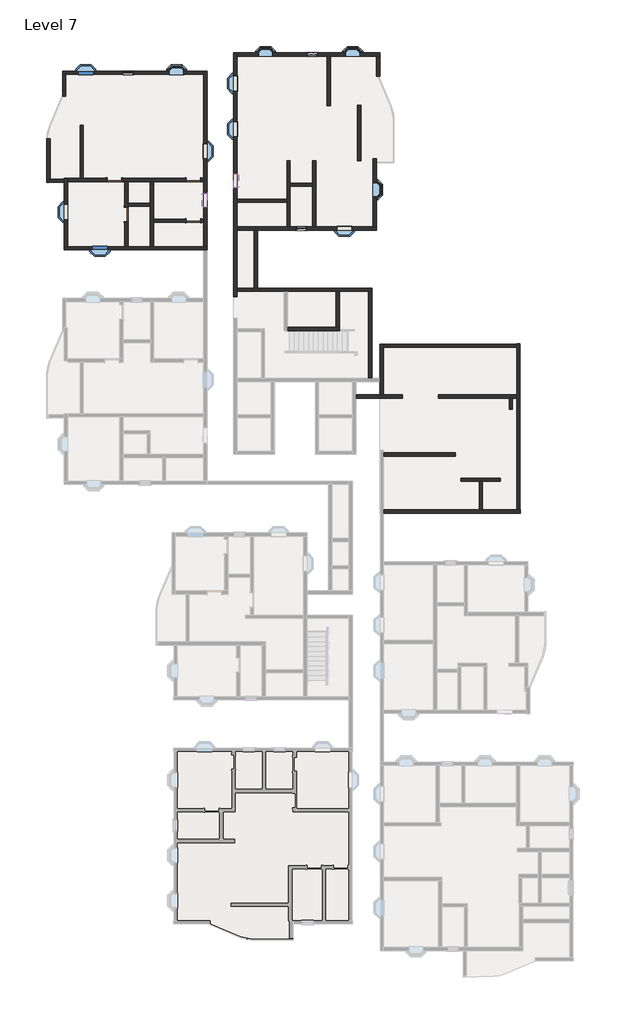
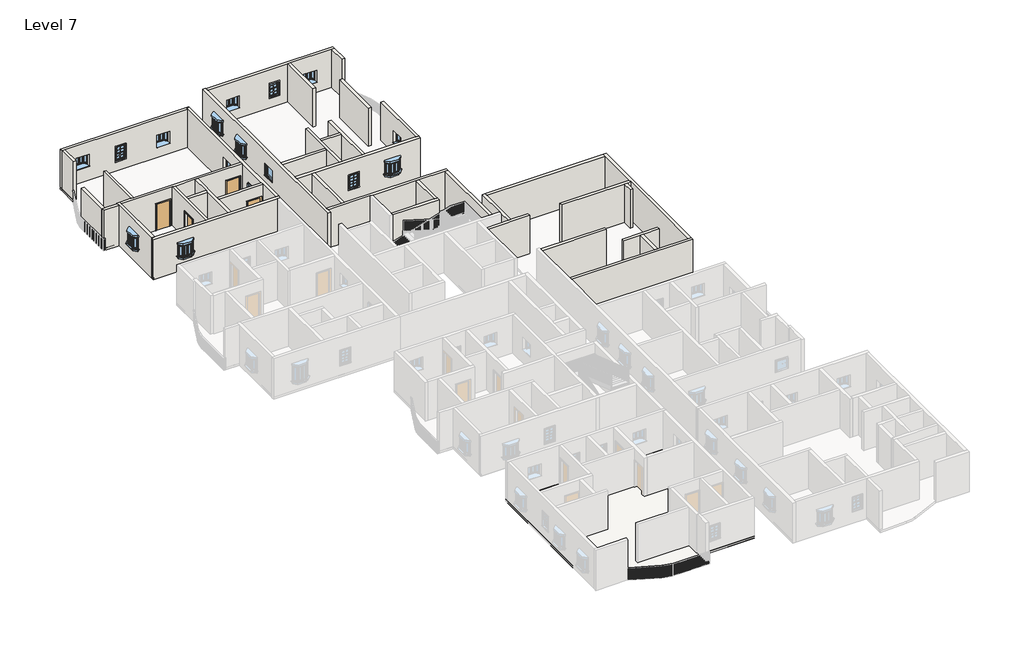
# One storey, part 4 of 14: 39 walls, 16 windows, 4 doors, 2 roofs.
# Revit data of these elements (continued)
# Elements 31, 45 (IfcWall, "9\" w") (continued)
#   wall height = 10' - 0"
#   Phase Created = New Construction
#   Base Constraint = Level 7
#   Top Constraint = Level 8
#   Materials on its faces: "Default Wall", "Brick, Soldier Course"
# Element 32 (IfcWall, "9\" w")
#   Top Offset = 0' - 0"
#   Base Offset = 0' - 0"
#   wall height = 10' - 0"
#   Phase Created = New Construction
#   Base Constraint = Level 7
#   Top Constraint = Level 8
#   Materials on its faces: "Default Wall", "Grass"
# Element 33 (IfcWall, "9\" w")
#   Top Offset = 0' - 0"
#   Base Offset = 0' - 0"
#   wall height = 10' - 0"
#   Phase Created = New Construction
#   Base Constraint = Level 7
#   Top Constraint = Level 8
#   Materials on its faces: "Default Wall", "Brick, Soldier Course", "Earth"
# Element 34 (IfcWall, "9\" w")
#   Top Offset = 0' - 0"
#   Base Offset = 0' - 0"
#   wall height = 10' - 0"
#   Phase Created = New Construction
#   Base Constraint = Level 7
#   Top Constraint = Level 8
#   Materials on its faces: "Default Wall", "Earth"
# Element 35 (IfcWall, "9\" w")
#   Top Offset = 0' - 0"
#   Base Offset = 0' - 0"
#   wall height = 10' - 0"
#   Phase Created = New Construction
#   Base Constraint = Level 7
#   Top Constraint = Level 8
#   Materials on its faces: "Default Wall", "Parking Stripe"
# Elements 36, 37, 38 (IfcWall, "9\" w")
#   Top Offset = 0' - 0"
#   Base Offset = 0' - 0"
#   wall height = 10' - 0"
#   Phase Created = New Construction
#   Base Constraint = Level 7
#   Top Constraint = Level 8
#   Materials on its faces: "Default Wall", "Window Frame"
# Element 43 (IfcWall, "9\" w")
#   Top Offset = 0' - 0"
#   Base Offset = 0' - 0"
#   wall height = 10' - 0"
#   Phase Created = New Construction
#   Base Constraint = Level 7
#   Top Constraint = Level 8
#   Materials on its faces: "Default Wall", "Parking Stripe", "Default Mass Interior Wall"
# Element 44 (IfcWall, "9\" w")
#   Top Offset = 0' - 0"
#   Base Offset = 0' - 0"
#   wall height = 10' - 0"
#   Phase Created = New Construction
#   Base Constraint = Level 7
#   Top Constraint = Level 8
#   Materials on its faces: "Default Wall", "Parking Stripe", "Brick, Soldier Course"
# Element 46 (IfcWindow, "910x910mm")
#   Mark = "362"
#   Phase Created = New Construction
#   Materials on its faces: "Window Frame", "Glass"
# Element 47 (IfcWindow, "910x910mm")
#   Mark = "363"
#   Phase Created = New Construction
#   Materials on its faces: "Window Frame", "Glass"
# Element 48 (IfcWindow, "910x910mm")
#   Mark = "364"
#   Phase Created = New Construction
#   Materials on its faces: "Window Frame", "Glass"
# Element 49 (IfcWindow, "910x910mm")
#   Mark = "394"
#   Phase Created = New Construction
#   Materials on its faces: "Window Frame", "Glass"
# Element 50 (IfcWindow, "910x910mm")
#   Mark = "395"
#   Phase Created = New Construction
#   Materials on its faces: "Window Frame", "Glass"
# Element 51 (IfcWindow, "910x910mm")
#   Mark = "475"
#   Phase Created = New Construction
#   Materials on its faces: "Window Frame", "Glass"
# Element 52 (IfcWindow, "910x910mm")
#   Mark = "476"
#   Phase Created = New Construction
#   Materials on its faces: "Window Frame", "Glass"
# Element 53 (IfcWindow, "910x910mm")
#   Mark = "484"
#   Phase Created = New Construction
#   Materials on its faces: "Window Frame", "Glass"
# Element 54 (IfcWindow, "910x910mm")
#   Mark = "485"
#   Phase Created = New Construction
#   Materials on its faces: "Window Frame", "Glass"
# Element 55 (IfcWindow, "910x910mm")
#   Mark = "396"
#   Phase Created = New Construction
#   Materials on its faces: "Window Frame", "Glass"
# Element 56 (IfcWindow, "910x910mm")
#   Mark = "397"
#   Phase Created = New Construction
#   Materials on its faces: "Window Frame", "Glass"
# Element 57 (IfcWindow, "Window-Double-Hung : 26\" x 42\"")
#   Mark = "477"
#   Window Inset = 0' - 0"
#   Interior Wall Closure = 0' - 1 1/2"
#   Frame Extension = 0' - 1 1/4"
#   Exterior Wall Closure = 0' - 0 1/2"
#   Interior Trim Visibility = yes
#   Indicator Visibility = yes
#   Exterior Trim Visibility = yes
#   Phase Created = New Construction
#   Materials on its faces: "Wood - Stained", "Glass", "Clad - White"
# Element 58 (IfcWindow, "Window-Double-Hung : 26\" x 42\"")
#   Mark = "486"
#   Window Inset = 0' - 0"
#   Interior Wall Closure = 0' - 1 1/2"
#   Frame Extension = 0' - 1 1/4"
#   Exterior Wall Closure = 0' - 0 1/2"
#   Interior Trim Visibility = yes
#   Indicator Visibility = yes
#   Exterior Trim Visibility = yes
#   Phase Created = New Construction
#   Materials on its faces: "Wood - Stained", "Glass", "Clad - White"
# Element 59 (IfcWindow, "Window-Double-Hung : 26\" x 42\"")
#   Mark = "415"
#   Window Inset = 0' - 0"
#   Interior Wall Closure = 0' - 1 1/2"
#   Frame Extension = 0' - 1 1/4"
#   Exterior Wall Closure = 0' - 0 1/2"
#   Interior Trim Visibility = yes
#   Indicator Visibility = yes
#   Exterior Trim Visibility = yes
#   Phase Created = New Construction
#   Materials on its faces: "Wood - Stained", "Glass", "Clad - White"
# Element 60 (IfcWindow, "Windows_Sgl_w-Glazing_Bars : 910x910mm")
#   Mark = "398"
#   Phase Created = New Construction
#   Materials on its faces: "Window Frame", "Glass"
# Element 61 (IfcWindow, "Windows_Sgl_w-Glazing_Bars : 910x910mm")
#   Mark = "402"
#   Phase Created = New Construction
#   Materials on its faces: "Window Frame", "Glass"
# Materials
#   "Door - Panel": class "Wood", colour RGB 210 159 95, transparency 0, Cost = 0
#   "Door - Frame": colour RGB 118 70 51, transparency 0, Cost = 0
#   "Window Frame": colour RGB 249 249 249, transparency 0
#   "Glass": class "Glass", colour RGB 0 128 192, transparency 0.75, Description = "Soda Lime Glass", Cost = 0
#   "Wood - Stained": class "Wood", colour RGB 224 178 126, transparency 0, Cost = 0
#   "Clad - White": class "Wood", colour RGB 242 242 238, transparency 0, Cost = 0
#   "Default Roof": colour RGB 88 101 114, transparency 0, Cost = 0
#   "Carpet (1)": class "Carpet", colour RGB 124 80 67, transparency 0, Description = "Interior finish", Cost = 0
#   "Default Wall": colour RGB 128 128 128, transparency 0, Cost = 0
#   "Grass": class "Generic", colour RGB 104 137 66, transparency 0, Description = "Physical material.", Cost = 0
#   "Parking Stripe": class "Paint", colour RGB 250 250 91, transparency 0, Cost = 0
#   "Brick, Soldier Course": class "Masonry", colour RGB 170 98 104, transparency 0, Description = "Common brick soldier coursed", Cost = 0
#   "Default Mass Interior Wall": class "Generic", colour RGB 195 229 126, transparency 0, Cost = 0
#   "Earth": class "Generic", colour RGB 97 75 62, transparency 0, Description = "Soil", Cost = 0
